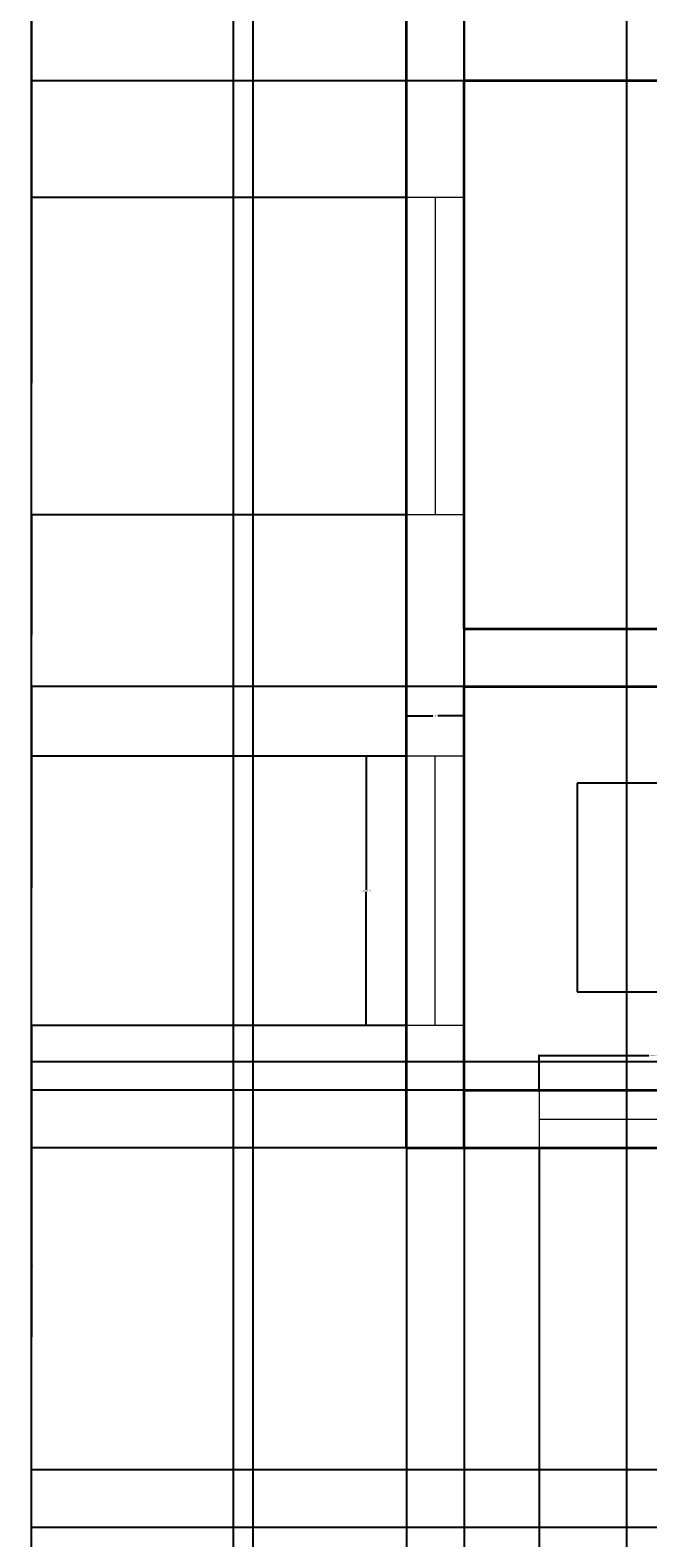
# Model space of a CAD drawing. Units: inches. Extents: x 2863 to 3499, y 1212 to 2136.
# Tile 2 of 7: x 2863 to 2991, y 1372 to 1686. Entities that reach past the tile are written whole.
import ezdxf

# ---------------------------------------------------------------- set-up
doc = ezdxf.new("R2010")
doc.units = ezdxf.units.IN
doc.linetypes.add('DASHED2', pattern=[9.525, 6.35, -3.175])
for name, color, linetype, lineweight in [('A-ANNO-DIMS', 2, 'Continuous', 18), ('A-FLOR-OVHD', 51, 'DASHED2', 18), ('A-FLOR-STRS', 51, 'Continuous', 25), ('A-GLAZ', 191, 'Continuous', 18), ('A-WALL', 51, 'Continuous', 35), ('C-PROP', 51, 'Continuous', 25)]:
    doc.layers.add(name, color=color, linetype=linetype, lineweight=lineweight)
doc.styles.get("Standard").update_dxf_attribs({"font": 'arial.ttf'})
doc.dimstyles.get("Standard").update_dxf_attribs({"dimtxt": 0.18, "dimasz": 0.18, "dimexe": 0.18, "dimexo": 0.0625, "dimgap": 0.09, "dimtad": 0, "dimtih": 1, "dimtoh": 1, "dimdec": 4, "dimzin": 0, "dimdsep": 46, "dimtxsty": 'Standard', "dimcen": 0.09, "dimadec": 0, "dimazin": 0, "dimtfac": 1, "dimtdec": 4, "dimtofl": 0, "dimtmove": 0, "dimatfit": 3, "dimfxl": 1, "dimtolj": 1, "dimtzin": 0, "dimarcsym": 0})

# ---------------------------------------------------------------- blocks, each defined once
blk = doc.blocks.new('WINDOW-48IN')
for p, q in [((12, 48), (0, 48)), ((6, 48), (6, 0)), ((12, 0), (0, 0))]:
    blk.add_line(p, q)
blk = doc.blocks.new('WINDOW-56IN')
for p, q in [((12, 56), (0, 56)), ((6, 0), (6, 56)), ((12, 0), (0, 0))]:
    blk.add_line(p, q)
blk = doc.blocks.new('*D33')
at = {"layer": 'A-ANNO-DIMS', "color": 0, "lineweight": -2, "transparency": 16777216}
for p, q in [((2968.53, 1465.23), (2968.53, 1472.55)), ((2968.71, 1472.37), (2991.41, 1472.37)), ((3016.35, 1472.37), (2993.64, 1472.37)), ((3016.53, 1465.23), (3016.53, 1472.55))]:
    blk.add_line(p, q, dxfattribs=at)
at = {"layer": 'A-ANNO-DIMS', "color": 0, "transparency": 16777216}
for points in [[(2968.71, 1472.4), (2968.71, 1472.34), (2968.53, 1472.37)], [(3016.35, 1472.4), (3016.35, 1472.34), (3016.53, 1472.37)]]:
    blk.add_solid(points, dxfattribs=at)
at = {"layer": 'Defpoints', "color": 0, "transparency": 16777216}
for p in [(2968.53, 1472.37), (2968.53, 1465.17), (3016.53, 1465.17)]:
    blk.add_point(p, dxfattribs=at)
at = {"layer": 'A-ANNO-DIMS', "color": 0, "transparency": 16777216, "insert": (2992.53, 1472.37), "char_height": 0.18, "attachment_point": 5}
blk.add_mtext('\\A1;WINDOW 48 TYP.', dxfattribs=at)
blk = doc.blocks.new('*D47')
at = {"layer": 'A-ANNO-DIMS', "color": 0, "lineweight": -2, "transparency": 16777216}
for p, q in [((2940.85, 1534.65), (2932.34, 1534.65)), ((2932.52, 1534.47), (2932.52, 1506.83)), ((2932.52, 1478.83), (2932.52, 1506.46)), ((2940.85, 1478.65), (2932.34, 1478.65))]:
    blk.add_line(p, q, dxfattribs=at)
at = {"layer": 'A-ANNO-DIMS', "color": 0, "transparency": 16777216}
for points in [[(2932.49, 1534.47), (2932.55, 1534.47), (2932.52, 1534.65)], [(2932.49, 1478.83), (2932.55, 1478.83), (2932.52, 1478.65)]]:
    blk.add_solid(points, dxfattribs=at)
at = {"layer": 'Defpoints', "color": 0, "transparency": 16777216}
for p in [(2932.52, 1534.65), (2940.92, 1534.65), (2940.92, 1478.65)]:
    blk.add_point(p, dxfattribs=at)
at = {"layer": 'A-ANNO-DIMS', "color": 0, "transparency": 16777216, "insert": (2932.52, 1506.65), "char_height": 0.18, "attachment_point": 5}
blk.add_mtext('\\A1;WINDOW 56 TYP.', dxfattribs=at)
blk = doc.blocks.new('*D48')
at = {"layer": 'A-ANNO-DIMS', "color": 0, "lineweight": -2, "transparency": 16777216}
for p, q in [((2940.92, 1534.71), (2940.92, 1543.23)), ((2941.1, 1543.05), (2946.4, 1543.05)), ((2952.74, 1543.05), (2947.44, 1543.05)), ((2952.92, 1534.71), (2952.92, 1543.23))]:
    blk.add_line(p, q, dxfattribs=at)
at = {"layer": 'A-ANNO-DIMS', "color": 0, "transparency": 16777216}
for points in [[(2941.1, 1543.08), (2941.1, 1543.02), (2940.92, 1543.05)], [(2952.74, 1543.08), (2952.74, 1543.02), (2952.92, 1543.05)]]:
    blk.add_solid(points, dxfattribs=at)
at = {"layer": 'Defpoints', "color": 0, "transparency": 16777216}
for p in [(2952.92, 1543.05), (2940.92, 1534.65), (2952.92, 1534.65)]:
    blk.add_point(p, dxfattribs=at)
at = {"layer": 'A-ANNO-DIMS', "color": 0, "transparency": 16777216, "insert": (2946.92, 1543.05), "char_height": 0.18, "attachment_point": 5}
blk.add_mtext('\\A1;12 TYP.', dxfattribs=at)
blk = doc.blocks.new('*D50')
at = {"layer": 'A-ANNO-DIMS', "color": 0, "lineweight": -2, "transparency": 16777216}
for p, q in [((2904.85, 2094.17), (2862.72, 2094.17)), ((2862.9, 2093.99), (2862.9, 1674.35)), ((2862.9, 1254.35), (2862.9, 1673.98)), ((2904.85, 1254.17), (2862.72, 1254.17))]:
    blk.add_line(p, q, dxfattribs=at)
at = {"layer": 'A-ANNO-DIMS', "color": 0, "transparency": 16777216}
for points in [[(2862.87, 2093.99), (2862.93, 2093.99), (2862.9, 2094.17)], [(2862.87, 1254.35), (2862.93, 1254.35), (2862.9, 1254.17)]]:
    blk.add_solid(points, dxfattribs=at)
at = {"layer": 'Defpoints', "color": 0, "transparency": 16777216}
for p in [(2862.9, 2094.17), (2904.92, 2094.17), (2904.92, 1254.17)]:
    blk.add_point(p, dxfattribs=at)
at = {"layer": 'A-ANNO-DIMS', "color": 0, "transparency": 16777216, "insert": (2862.9, 1674.17), "char_height": 0.18, "attachment_point": 5}
blk.add_mtext('\\A1;840', dxfattribs=at)
blk = doc.blocks.new('*D64')
at = {"layer": 'A-ANNO-DIMS', "color": 0, "lineweight": -2, "transparency": 16777216}
for p, q in [((2952.85, 1549.17), (2862.72, 1549.17)), ((2862.9, 1548.99), (2862.9, 1507.35)), ((2862.9, 1465.35), (2862.9, 1506.98)), ((2952.85, 1465.17), (2862.72, 1465.17))]:
    blk.add_line(p, q, dxfattribs=at)
at = {"layer": 'A-ANNO-DIMS', "color": 0, "transparency": 16777216}
for points in [[(2862.87, 1548.99), (2862.93, 1548.99), (2862.9, 1549.17)], [(2862.87, 1465.35), (2862.93, 1465.35), (2862.9, 1465.17)]]:
    blk.add_solid(points, dxfattribs=at)
at = {"layer": 'Defpoints', "color": 0, "transparency": 16777216}
for p in [(2862.9, 1549.17), (2952.92, 1549.17), (2952.92, 1465.17)]:
    blk.add_point(p, dxfattribs=at)
at = {"layer": 'A-ANNO-DIMS', "color": 0, "transparency": 16777216, "insert": (2862.9, 1507.17), "char_height": 0.18, "attachment_point": 5}
blk.add_mtext('\\A1;84', dxfattribs=at)
blk = doc.blocks.new('*D65')
at = {"layer": 'A-ANNO-DIMS', "color": 0, "lineweight": -2, "transparency": 16777216}
for p, q in [((2952.85, 1675.17), (2862.72, 1675.17)), ((2862.9, 1674.99), (2862.9, 1612.35)), ((2862.9, 1549.35), (2862.9, 1611.98)), ((2952.85, 1549.17), (2862.72, 1549.17))]:
    blk.add_line(p, q, dxfattribs=at)
at = {"layer": 'A-ANNO-DIMS', "color": 0, "transparency": 16777216}
for points in [[(2862.87, 1674.99), (2862.93, 1674.99), (2862.9, 1675.17)], [(2862.87, 1549.35), (2862.93, 1549.35), (2862.9, 1549.17)]]:
    blk.add_solid(points, dxfattribs=at)
at = {"layer": 'Defpoints', "color": 0, "transparency": 16777216}
for p in [(2862.9, 1675.17), (2952.92, 1675.17), (2952.92, 1549.17)]:
    blk.add_point(p, dxfattribs=at)
at = {"layer": 'A-ANNO-DIMS', "color": 0, "transparency": 16777216, "insert": (2862.9, 1612.17), "char_height": 0.18, "attachment_point": 5}
blk.add_mtext('\\A1;126', dxfattribs=at)
blk = doc.blocks.new('*D66')
at = {"layer": 'A-ANNO-DIMS', "color": 0, "lineweight": -2, "transparency": 16777216}
for p, q in [((2952.85, 1800.17), (2862.72, 1800.17)), ((2862.9, 1799.99), (2862.9, 1737.85)), ((2862.9, 1675.35), (2862.9, 1737.48)), ((2952.85, 1675.17), (2862.72, 1675.17))]:
    blk.add_line(p, q, dxfattribs=at)
at = {"layer": 'A-ANNO-DIMS', "color": 0, "transparency": 16777216}
for points in [[(2862.87, 1799.99), (2862.93, 1799.99), (2862.9, 1800.17)], [(2862.87, 1675.35), (2862.93, 1675.35), (2862.9, 1675.17)]]:
    blk.add_solid(points, dxfattribs=at)
at = {"layer": 'Defpoints', "color": 0, "transparency": 16777216}
for p in [(2862.9, 1800.17), (2952.92, 1800.17), (2952.92, 1675.17)]:
    blk.add_point(p, dxfattribs=at)
at = {"layer": 'A-ANNO-DIMS', "color": 0, "transparency": 16777216, "insert": (2862.9, 1737.67), "char_height": 0.18, "attachment_point": 5}
blk.add_mtext('\\A1;125', dxfattribs=at)
blk = doc.blocks.new('*D69')
at = {"layer": 'A-ANNO-DIMS', "color": 0, "lineweight": -2, "transparency": 16777216}
for p, q in [((3204.85, 1453.17), (2862.72, 1453.17)), ((2862.9, 1452.99), (2862.9, 1413.85)), ((2862.9, 1374.35), (2862.9, 1413.48)), ((3204.85, 1374.17), (2862.72, 1374.17))]:
    blk.add_line(p, q, dxfattribs=at)
at = {"layer": 'A-ANNO-DIMS', "color": 0, "transparency": 16777216}
for points in [[(2862.87, 1452.99), (2862.93, 1452.99), (2862.9, 1453.17)], [(2862.87, 1374.35), (2862.93, 1374.35), (2862.9, 1374.17)]]:
    blk.add_solid(points, dxfattribs=at)
at = {"layer": 'Defpoints', "color": 0, "transparency": 16777216}
for p in [(3204.92, 1453.17), (2862.9, 1374.17), (3204.92, 1374.17)]:
    blk.add_point(p, dxfattribs=at)
at = {"layer": 'A-ANNO-DIMS', "color": 0, "transparency": 16777216, "insert": (2862.9, 1413.67), "char_height": 0.18, "attachment_point": 5}
blk.add_mtext('\\A1;79', dxfattribs=at)
blk = doc.blocks.new('*D70')
at = {"layer": 'A-ANNO-DIMS', "color": 0, "lineweight": -2, "transparency": 16777216}
for p, q in [((2940.92, 1453.1), (2940.92, 1211.97)), ((3204.92, 1374.1), (3204.92, 1211.97)), ((2941.1, 1212.15), (3072.63, 1212.15)), ((3204.74, 1212.15), (3073.21, 1212.15))]:
    blk.add_line(p, q, dxfattribs=at)
at = {"layer": 'A-ANNO-DIMS', "color": 0, "transparency": 16777216}
for points in [[(2941.1, 1212.18), (2941.1, 1212.12), (2940.92, 1212.15)], [(3204.74, 1212.18), (3204.74, 1212.12), (3204.92, 1212.15)]]:
    blk.add_solid(points, dxfattribs=at)
at = {"layer": 'Defpoints', "color": 0, "transparency": 16777216}
for p in [(2940.92, 1453.17), (3204.92, 1374.17), (3204.92, 1212.15)]:
    blk.add_point(p, dxfattribs=at)
at = {"layer": 'A-ANNO-DIMS', "color": 0, "transparency": 16777216, "insert": (3072.92, 1212.15), "char_height": 0.18, "attachment_point": 5}
blk.add_mtext('\\A1;264', dxfattribs=at)
blk = doc.blocks.new('*D74')
at = {"layer": 'A-ANNO-DIMS', "color": 0, "lineweight": -2, "transparency": 16777216}
for p, q in [((3408.85, 1471.09), (2862.72, 1471.09)), ((2862.9, 1470.91), (2862.9, 1428.81)), ((2862.9, 1386.35), (2862.9, 1428.44)), ((3408.85, 1386.17), (2862.72, 1386.17))]:
    blk.add_line(p, q, dxfattribs=at)
at = {"layer": 'A-ANNO-DIMS', "color": 0, "transparency": 16777216}
for points in [[(2862.87, 1470.91), (2862.93, 1470.91), (2862.9, 1471.09)], [(2862.87, 1386.35), (2862.93, 1386.35), (2862.9, 1386.17)]]:
    blk.add_solid(points, dxfattribs=at)
at = {"layer": 'Defpoints', "color": 0, "transparency": 16777216}
for p in [(3408.92, 1471.09), (2862.9, 1386.17), (3408.92, 1386.17)]:
    blk.add_point(p, dxfattribs=at)
at = {"layer": 'A-ANNO-DIMS', "color": 0, "transparency": 16777216, "insert": (2862.9, 1428.63), "char_height": 0.18, "attachment_point": 5}
blk.add_mtext('\\A1;84.92', dxfattribs=at)
blk = doc.blocks.new('*D76')
at = {"layer": 'A-ANNO-DIMS', "color": 0, "lineweight": -2, "transparency": 16777216}
for p, q in [((2952.92, 1675.1), (2952.92, 1211.97)), ((3121.92, 1675.1), (3121.92, 1211.97)), ((2953.1, 1212.15), (3037.14, 1212.15)), ((3121.74, 1212.15), (3037.7, 1212.15))]:
    blk.add_line(p, q, dxfattribs=at)
at = {"layer": 'A-ANNO-DIMS', "color": 0, "transparency": 16777216}
for points in [[(2953.1, 1212.18), (2953.1, 1212.12), (2952.92, 1212.15)], [(3121.74, 1212.18), (3121.74, 1212.12), (3121.92, 1212.15)]]:
    blk.add_solid(points, dxfattribs=at)
at = {"layer": 'Defpoints', "color": 0, "transparency": 16777216}
for p in [(2952.92, 1675.17), (3121.92, 1675.17), (3121.92, 1212.15)]:
    blk.add_point(p, dxfattribs=at)
at = {"layer": 'A-ANNO-DIMS', "color": 0, "transparency": 16777216, "insert": (3037.42, 1212.15), "char_height": 0.18, "attachment_point": 5}
blk.add_mtext('\\A1;169', dxfattribs=at)
blk = doc.blocks.new('*D83')
at = {"layer": 'A-ANNO-DIMS', "color": 0, "lineweight": -2, "transparency": 16777216}
for p, q in [((2940.85, 1478.65), (2862.72, 1478.65)), ((2862.9, 1478.47), (2862.9, 1466.09)), ((2862.9, 1453.35), (2862.9, 1465.72)), ((2940.85, 1453.17), (2862.72, 1453.17))]:
    blk.add_line(p, q, dxfattribs=at)
at = {"layer": 'A-ANNO-DIMS', "color": 0, "transparency": 16777216}
for points in [[(2862.87, 1478.47), (2862.93, 1478.47), (2862.9, 1478.65)], [(2862.87, 1453.35), (2862.93, 1453.35), (2862.9, 1453.17)]]:
    blk.add_solid(points, dxfattribs=at)
at = {"layer": 'Defpoints', "color": 0, "transparency": 16777216}
for p in [(2862.9, 1478.65), (2940.92, 1478.65), (2940.92, 1453.17)]:
    blk.add_point(p, dxfattribs=at)
at = {"layer": 'A-ANNO-DIMS', "color": 0, "transparency": 16777216, "insert": (2862.9, 1465.91), "char_height": 0.18, "attachment_point": 5}
blk.add_mtext('\\A1;25.48', dxfattribs=at)
blk = doc.blocks.new('*D84')
at = {"layer": 'A-ANNO-DIMS', "color": 0, "lineweight": -2, "transparency": 16777216}
for p, q in [((2940.85, 1584.91), (2862.72, 1584.91)), ((2862.9, 1584.73), (2862.9, 1559.96)), ((2862.9, 1534.83), (2862.9, 1559.6)), ((2940.85, 1534.65), (2862.72, 1534.65))]:
    blk.add_line(p, q, dxfattribs=at)
at = {"layer": 'A-ANNO-DIMS', "color": 0, "transparency": 16777216}
for points in [[(2862.87, 1584.73), (2862.93, 1584.73), (2862.9, 1584.91)], [(2862.87, 1534.83), (2862.93, 1534.83), (2862.9, 1534.65)]]:
    blk.add_solid(points, dxfattribs=at)
at = {"layer": 'Defpoints', "color": 0, "transparency": 16777216}
for p in [(2862.9, 1584.91), (2940.92, 1584.91), (2940.92, 1534.65)]:
    blk.add_point(p, dxfattribs=at)
at = {"layer": 'A-ANNO-DIMS', "color": 0, "transparency": 16777216, "insert": (2862.9, 1559.78), "char_height": 0.18, "attachment_point": 5}
blk.add_mtext('\\A1;50.26', dxfattribs=at)
blk = doc.blocks.new('*D85')
at = {"layer": 'A-ANNO-DIMS', "color": 0, "lineweight": -2, "transparency": 16777216}
for p, q in [((2940.85, 1650.91), (2862.72, 1650.91)), ((2862.9, 1650.73), (2862.9, 1618.09)), ((2862.9, 1585.09), (2862.9, 1617.73)), ((2940.85, 1584.91), (2862.72, 1584.91))]:
    blk.add_line(p, q, dxfattribs=at)
at = {"layer": 'A-ANNO-DIMS', "color": 0, "transparency": 16777216}
for points in [[(2862.87, 1650.73), (2862.93, 1650.73), (2862.9, 1650.91)], [(2862.87, 1585.09), (2862.93, 1585.09), (2862.9, 1584.91)]]:
    blk.add_solid(points, dxfattribs=at)
at = {"layer": 'Defpoints', "color": 0, "transparency": 16777216}
for p in [(2862.9, 1650.91), (2940.92, 1650.91), (2940.92, 1584.91)]:
    blk.add_point(p, dxfattribs=at)
at = {"layer": 'A-ANNO-DIMS', "color": 0, "transparency": 16777216, "insert": (2862.9, 1617.91), "char_height": 0.18, "attachment_point": 5}
blk.add_mtext('\\A1;66', dxfattribs=at)
blk = doc.blocks.new('*D86')
at = {"layer": 'A-ANNO-DIMS', "color": 0, "lineweight": -2, "transparency": 16777216}
for p, q in [((2940.85, 1728.91), (2862.72, 1728.91)), ((2862.9, 1728.73), (2862.9, 1690.09)), ((2862.9, 1651.09), (2862.9, 1689.73)), ((2940.85, 1650.91), (2862.72, 1650.91))]:
    blk.add_line(p, q, dxfattribs=at)
at = {"layer": 'A-ANNO-DIMS', "color": 0, "transparency": 16777216}
for points in [[(2862.87, 1728.73), (2862.93, 1728.73), (2862.9, 1728.91)], [(2862.87, 1651.09), (2862.93, 1651.09), (2862.9, 1650.91)]]:
    blk.add_solid(points, dxfattribs=at)
at = {"layer": 'Defpoints', "color": 0, "transparency": 16777216}
for p in [(2862.9, 1728.91), (2940.92, 1728.91), (2940.92, 1650.91)]:
    blk.add_point(p, dxfattribs=at)
at = {"layer": 'A-ANNO-DIMS', "color": 0, "transparency": 16777216, "insert": (2862.9, 1689.91), "char_height": 0.18, "attachment_point": 5}
blk.add_mtext('\\A1;78', dxfattribs=at)
blk = doc.blocks.new('*D101')
at = {"layer": 'A-ANNO-DIMS', "color": 0, "lineweight": -2, "transparency": 16777216}
for p, q in [((2940.92, 1453.1), (2940.92, 1211.97)), ((2968.53, 1453.1), (2968.53, 1211.97)), ((2941.1, 1212.15), (2954.34, 1212.15)), ((2968.35, 1212.15), (2955.1, 1212.15))]:
    blk.add_line(p, q, dxfattribs=at)
at = {"layer": 'A-ANNO-DIMS', "color": 0, "transparency": 16777216}
for points in [[(2941.1, 1212.18), (2941.1, 1212.12), (2940.92, 1212.15)], [(2968.35, 1212.18), (2968.35, 1212.12), (2968.53, 1212.15)]]:
    blk.add_solid(points, dxfattribs=at)
at = {"layer": 'Defpoints', "color": 0, "transparency": 16777216}
for p in [(2940.92, 1453.17), (2968.53, 1453.17), (2968.53, 1212.15)]:
    blk.add_point(p, dxfattribs=at)
at = {"layer": 'A-ANNO-DIMS', "color": 0, "transparency": 16777216, "insert": (2954.72, 1212.15), "char_height": 0.18, "attachment_point": 5}
blk.add_mtext('\\A1;27.61', dxfattribs=at)
blk = doc.blocks.new('*D111')
at = {"layer": 'A-ANNO-DIMS', "color": 0, "lineweight": -2, "transparency": 16777216}
for p, q in [((2952.92, 1549.23), (2952.92, 2136.37)), ((2997.55, 1549.23), (2997.55, 2136.37)), ((2953.1, 2136.19), (2974.83, 2136.19)), ((2997.37, 2136.19), (2975.63, 2136.19))]:
    blk.add_line(p, q, dxfattribs=at)
at = {"layer": 'A-ANNO-DIMS', "color": 0, "transparency": 16777216}
for points in [[(2953.1, 2136.22), (2953.1, 2136.16), (2952.92, 2136.19)], [(2997.37, 2136.22), (2997.37, 2136.16), (2997.55, 2136.19)]]:
    blk.add_solid(points, dxfattribs=at)
at = {"layer": 'Defpoints', "color": 0, "transparency": 16777216}
for p in [(2997.55, 2136.19), (2952.92, 1549.17), (2997.55, 1549.17)]:
    blk.add_point(p, dxfattribs=at)
at = {"layer": 'A-ANNO-DIMS', "color": 0, "transparency": 16777216, "insert": (2975.23, 2136.19), "char_height": 0.18, "attachment_point": 5}
blk.add_mtext('\\A1;44.63', dxfattribs=at)
blk = doc.blocks.new('*D112')
at = {"layer": 'A-ANNO-DIMS', "color": 0, "lineweight": -2, "transparency": 16777216}
for p, q in [((2952.92, 1800.1), (2952.92, 1211.97)), ((2986.74, 1800.1), (2986.74, 1211.97)), ((2953.1, 1212.15), (2969.37, 1212.15)), ((2986.56, 1212.15), (2970.29, 1212.15))]:
    blk.add_line(p, q, dxfattribs=at)
at = {"layer": 'A-ANNO-DIMS', "color": 0, "transparency": 16777216}
for points in [[(2953.1, 1212.18), (2953.1, 1212.12), (2952.92, 1212.15)], [(2986.56, 1212.18), (2986.56, 1212.12), (2986.74, 1212.15)]]:
    blk.add_solid(points, dxfattribs=at)
at = {"layer": 'Defpoints', "color": 0, "transparency": 16777216}
for p in [(2952.92, 1800.17), (2986.74, 1800.17), (2986.74, 1212.15)]:
    blk.add_point(p, dxfattribs=at)
at = {"layer": 'A-ANNO-DIMS', "color": 0, "transparency": 16777216, "insert": (2969.83, 1212.15), "char_height": 0.18, "attachment_point": 5}
blk.add_mtext('\\A1;33.825', dxfattribs=at)

msp = doc.modelspace()

# ---------------------------------------------------------------- linework, layer by layer
at = {"layer": 'A-FLOR-OVHD'}
for p, q in [((2940.9168, 1374.1651), (2940.9168, 1453.1651)), ((2952.9168, 1453.1651), (2952.9168, 1386.1651)), ((2952.9168, 1386.1651), (3204.9168, 1386.1651)), ((3216.9168, 1374.1651), (2940.9168, 1374.1651))]:
    msp.add_line(p, q, dxfattribs=at)
at = {"layer": 'A-FLOR-STRS'}
for p, q in [((3105.5458, 1529.0656), (2976.4727, 1529.0656)), ((2976.4727, 1529.0656), (2976.4727, 1485.602)), ((2976.4727, 1485.602), (3105.5458, 1485.602))]:
    msp.add_line(p, q, dxfattribs=at)
at = {"layer": 'A-GLAZ'}
for p, q in [((2952.9168, 1650.9094), (2940.9168, 1650.9094)), ((2946.9168, 1650.9094), (2946.9168, 1584.9094)), ((2952.9168, 1584.9094), (2940.9168, 1584.9094))]:
    msp.add_line(p, q, dxfattribs=at)
at = {"layer": 'A-WALL'}
for p, q in [((3121.9168, 1675.1651), (2952.9168, 1675.1651)), ((2952.9168, 1561.1651), (2952.9168, 1675.1651)), ((2952.9168, 1561.1651), (3121.9168, 1561.1651)), ((2952.9168, 1453.1651), (2952.9168, 1549.1651)), ((2952.9168, 1549.1651), (3133.9168, 1549.1651)), ((2952.9168, 1465.1651), (3133.9168, 1465.1651)), ((2940.9168, 1453.1651), (3133.9168, 1453.1651))]:
    msp.add_line(p, q, dxfattribs=at)
msp.add_lwpolyline([(2940.9168, 1453.1651), (2940.9168, 2094.1651), (3420.9168, 2094.1651), (3420.9168, 1374.1651), (3216.9168, 1374.1651)], dxfattribs=at)
at = {"layer": 'C-PROP'}
for p, q in [((2904.9168, 1254.1651), (2904.9168, 2094.1651)), ((2908.9168, 2094.1651), (2908.9168, 1258.1651))]:
    msp.add_line(p, q, dxfattribs=at)

# ---------------------------------------------------------------- block references
at = {"layer": 'A-GLAZ'}
msp.add_blockref('WINDOW-56IN', (2940.917, 1478.646), dxfattribs=at)
at = {"layer": 'A-GLAZ', "rotation": 89.9999999999968}
msp.add_blockref('WINDOW-48IN', (3016.5255, 1453.1653), dxfattribs=at)

# ---------------------------------------------------------------- dimensions: what is measured, and where the dimension line sits
at = {"layer": 'A-ANNO-DIMS'}
for base, p1, p2, override, picture, middle in [((2997.5458, 2136.1851), (2952.9168, 1549.1651), (2997.5458, 1549.1651), {"dimdec": 2, "dimlfac": 1, "dimrnd": 0, "dimzin": 0, "dimdsep": 46, "dimlunit": 2}, '*D111', (2975.2313, 2136.1851)), ((2986.7418, 1212.1451), (2952.9168, 1800.1651), (2986.7418, 1800.1651), {"dimdec": 3, "dimlfac": 1, "dimrnd": 0, "dimzin": 0, "dimdsep": 46, "dimlunit": 2}, '*D112', (2969.8293, 1212.1451)), ((3121.9168, 1212.1451), (2952.9168, 1675.1651), (3121.9168, 1675.1651), {"dimdec": 0, "dimlfac": 1, "dimrnd": 0, "dimzin": 0, "dimdsep": 46, "dimlunit": 2}, '*D76', (3037.4168, 1212.1451)), ((3204.9168, 1212.1451), (2940.9168, 1453.1651), (3204.9168, 1374.1651), {"dimdec": 0, "dimlfac": 1, "dimrnd": 0, "dimzin": 0, "dimdsep": 46, "dimlunit": 2}, '*D70', (3072.9168, 1212.1451)), ((2968.5255, 1212.1451), (2940.9168, 1453.1651), (2968.5255, 1453.1651), {"dimdec": 2, "dimlfac": 1, "dimrnd": 0, "dimzin": 0, "dimdsep": 46, "dimlunit": 2}, '*D101', (2954.7211, 1212.1451))]:
    dim = msp.add_linear_dim(base=base, p1=p1, p2=p2, dimstyle='Standard', override=override, dxfattribs=at)
    dim.commit()
    dim.dimension.update_dxf_attribs({"geometry": picture, "text_midpoint": middle})
for base, p1, p2, override, picture, middle in [((2862.8968, 2094.1651), (2904.9168, 1254.1651), (2904.9168, 2094.1651), {"dimdec": 0, "dimlfac": 1, "dimrnd": 0, "dimzin": 0, "dimdsep": 46, "dimlunit": 2}, '*D50', (2862.8968, 1674.1651)), ((2862.8968, 1800.1651), (2952.9168, 1675.1651), (2952.9168, 1800.1651), {"dimdec": 0, "dimlfac": 1, "dimrnd": 0, "dimzin": 0, "dimdsep": 46, "dimlunit": 2}, '*D66', (2862.8968, 1737.6651)), ((2862.8968, 1728.9148), (2940.9168, 1650.9094), (2940.9168, 1728.9148), {"dimdec": 0, "dimlfac": 1, "dimrnd": 0, "dimzin": 0, "dimdsep": 46, "dimlunit": 2}, '*D86', (2862.8968, 1689.9121)), ((2862.8968, 1675.1651), (2952.9168, 1549.1651), (2952.9168, 1675.1651), {"dimdec": 0, "dimlfac": 1, "dimrnd": 0, "dimzin": 0, "dimdsep": 46, "dimlunit": 2}, '*D65', (2862.8968, 1612.1651)), ((2862.8968, 1650.9094), (2940.9168, 1584.9094), (2940.9168, 1650.9094), {"dimdec": 0, "dimlfac": 1, "dimrnd": 0, "dimzin": 0, "dimdsep": 46, "dimlunit": 2}, '*D85', (2862.8968, 1617.9094)), ((2862.8968, 1584.9094), (2940.9168, 1534.6455), (2940.9168, 1584.9094), {"dimdec": 2, "dimlfac": 1, "dimrnd": 0, "dimzin": 0, "dimdsep": 46, "dimlunit": 2}, '*D84', (2862.8968, 1559.7775)), ((2862.8968, 1549.1651), (2952.9168, 1465.1651), (2952.9168, 1549.1651), {"dimdec": 0, "dimlfac": 1, "dimrnd": 0, "dimzin": 0, "dimdsep": 46, "dimlunit": 2}, '*D64', (2862.8968, 1507.1651)), ((2862.8968, 1478.6455), (2940.9168, 1453.1651), (2940.9168, 1478.6455), {"dimdec": 2, "dimlfac": 1, "dimrnd": 0, "dimzin": 0, "dimdsep": 46, "dimlunit": 2}, '*D83', (2862.8968, 1465.9053)), ((2862.8968, 1386.1651), (3408.9168, 1471.0882), (3408.9168, 1386.1651), {"dimdec": 2, "dimlfac": 1, "dimrnd": 0, "dimzin": 0, "dimdsep": 46, "dimlunit": 2}, '*D74', (2862.8968, 1428.6266)), ((2862.8968, 1374.1651), (3204.9168, 1453.1651), (3204.9168, 1374.1651), {"dimdec": 0, "dimlfac": 1, "dimrnd": 0, "dimzin": 0, "dimdsep": 46, "dimlunit": 2}, '*D69', (2862.8968, 1413.6651))]:
    dim = msp.add_linear_dim(base=base, p1=p1, p2=p2, angle=90, dimstyle='Standard', override=override, dxfattribs=at)
    dim.commit()
    dim.dimension.update_dxf_attribs({"geometry": picture, "text_midpoint": middle})
dim = msp.add_linear_dim(base=(2952.9168, 1543.0455), p1=(2940.9168, 1534.6455), p2=(2952.9168, 1534.6455), text='<> TYP.', dimstyle='Standard', override={"dimdec": 0, "dimlfac": 1, "dimrnd": 0, "dimzin": 0, "dimdsep": 46, "dimlunit": 2}, dxfattribs=at)
dim.commit()
dim.dimension.update_dxf_attribs({"geometry": '*D48', "text_midpoint": (2946.9168, 1543.0455)})
for base, p1, p2, angle, picture, middle in [((2932.5168, 1534.6455), (2940.9168, 1478.6455), (2940.9168, 1534.6455), 90, '*D47', (2932.5168, 1506.6455)), ((2968.5255, 1472.3651), (3016.5255, 1465.1651), (2968.5255, 1465.1651), 180, '*D33', (2992.5255, 1472.3651))]:
    dim = msp.add_linear_dim(base=base, p1=p1, p2=p2, angle=angle, text='WINDOW <> TYP.', dimstyle='Standard', override={"dimdec": 0, "dimlfac": 1, "dimrnd": 0, "dimzin": 0, "dimdsep": 46, "dimlunit": 2}, dxfattribs=at)
    dim.commit()
    dim.dimension.update_dxf_attribs({"geometry": picture, "text_midpoint": middle})

doc.saveas('drawing.dxf')
